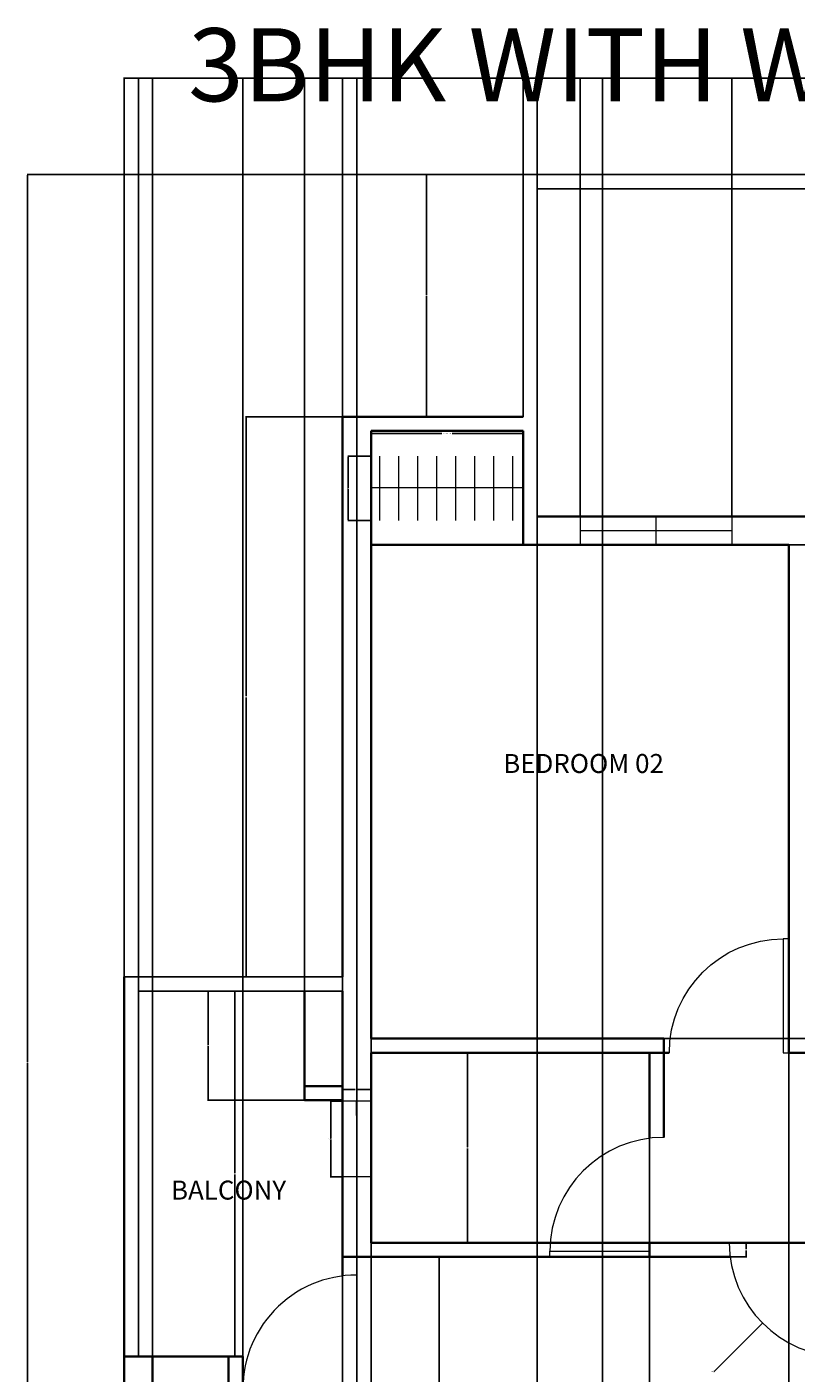
# Model space of a CAD drawing. Units: inches. Extents: x -83 to 475, y -99 to 539.
# Tile 2 of 3: x -83 to 160, y 114 to 539. Entities that reach past the tile are written whole.
import ezdxf

# ---------------------------------------------------------------- set-up
doc = ezdxf.new("R2010")
doc.units = ezdxf.units.IN
doc.header["$LTSCALE"] = 0.5
doc.header["$MEASUREMENT"] = 0
for name, color, linetype, lineweight in [('A-ANNO-DIMS', 2, 'Continuous', 18), ('A-ANNO-TEXT', 7, 'Continuous', 25), ('A-AREA-IDEN', 7, 'Continuous', 18), ('A-DOOR', 3, 'Continuous', 18), ('A-FURN', 8, 'Continuous', 13), ('A-GLAZ', 4, 'Continuous', 18), ('A-WALL', 7, 'Continuous', 35), ('A-WALL-PRPT', 7, 'Continuous', 25)]:
    doc.layers.add(name, color=color, linetype=linetype, lineweight=lineweight)
doc.styles.get("Standard").update_dxf_attribs({"font": 'arial.ttf'})
doc.dimstyles.get("Standard").update_dxf_attribs({"dimtxt": 0.18, "dimasz": 0.18, "dimexe": 0.18, "dimexo": 0.0625, "dimgap": 0.09, "dimtad": 0, "dimtih": 1, "dimtoh": 1, "dimdec": 4, "dimzin": 0, "dimdsep": 46, "dimtxsty": 'Standard', "dimcen": 0.09, "dimadec": 0, "dimazin": 0, "dimtfac": 1, "dimtdec": 4, "dimtofl": 0, "dimtmove": 0, "dimatfit": 3, "dimfxl": 1, "dimtolj": 1, "dimtzin": 0, "dimarcsym": 0})

# ---------------------------------------------------------------- blocks, each defined once
blk = doc.blocks.new('DOOR-SWING-36')
blk.add_lwpolyline([(1.78, 0), (0, 0), (0, 36.03), (1.78, 36.03)], close=True)
blk.add_arc((1.78, 0), 36, 0, 90)
blk = doc.blocks.new('WIN-48-TWO-LIGHT')
for p, q in [((0, 9), (0, 0)), ((24, 9), (24, 0)), ((48, 9), (48, 0)), ((0, 4.5), (48, 4.5))]:
    blk.add_line(p, q)
blk = doc.blocks.new('WIN-24')
for p, q in [((9, 24), (0, 24)), ((4.5, 19.41), (4.5, 24)), ((4.5, 19.41), (4.5, 0)), ((9, 0), (0, 0))]:
    blk.add_line(p, q)
blk = doc.blocks.new('WARDROBE-RAIL-48')
for p, q in [((2.64, 20.32), (2.64, 0)), ((8.64, 20.32), (8.64, 0)), ((14.64, 20.32), (14.64, 0)), ((20.64, 20.32), (20.64, 0)), ((26.64, 20.32), (26.64, 0)), ((32.64, 20.32), (32.64, 0)), ((38.64, 20.32), (38.64, 0)), ((44.64, 20.32), (44.64, 0)), ((48, 10.3), (0, 10.3))]:
    blk.add_line(p, q)
blk = doc.blocks.new('*D10')
at = {"layer": 'A-ANNO-DIMS', "color": 0, "lineweight": -2, "transparency": 16777216}
for p, q in [((16.39, 199.88), (12.67, 199.88)), ((12.85, 199.7), (12.85, 188.06)), ((12.85, 176.06), (12.85, 187.69)), ((16.39, 175.88), (12.67, 175.88))]:
    blk.add_line(p, q, dxfattribs=at)
at = {"layer": 'A-ANNO-DIMS', "color": 0, "transparency": 16777216}
for points in [[(12.82, 199.7), (12.88, 199.7), (12.85, 199.88)], [(12.82, 176.06), (12.88, 176.06), (12.85, 175.88)]]:
    blk.add_solid(points, dxfattribs=at)
at = {"layer": 'Defpoints', "color": 0, "transparency": 16777216}
for p in [(12.85, 199.88), (16.45, 199.88), (16.45, 175.88)]:
    blk.add_point(p, dxfattribs=at)
at = {"layer": 'A-ANNO-DIMS', "color": 0, "transparency": 16777216, "insert": (12.85, 187.88), "char_height": 0.18, "attachment_point": 5}
blk.add_mtext('\\A1;WINDOW 24 TYP.', dxfattribs=at)
blk = doc.blocks.new('*D11')
at = {"layer": 'A-ANNO-DIMS', "color": 0, "lineweight": -2, "transparency": 16777216}
for p, q in [((16.45, 199.94), (16.45, 203.66)), ((16.63, 203.48), (20.49, 203.48)), ((25.27, 203.48), (21.41, 203.48)), ((25.45, 199.94), (25.45, 203.66))]:
    blk.add_line(p, q, dxfattribs=at)
at = {"layer": 'A-ANNO-DIMS', "color": 0, "transparency": 16777216}
for points in [[(16.63, 203.51), (16.63, 203.45), (16.45, 203.48)], [(25.27, 203.51), (25.27, 203.45), (25.45, 203.48)]]:
    blk.add_solid(points, dxfattribs=at)
at = {"layer": 'Defpoints', "color": 0, "transparency": 16777216}
for p in [(25.45, 203.48), (16.45, 199.88), (25.45, 199.88)]:
    blk.add_point(p, dxfattribs=at)
at = {"layer": 'A-ANNO-DIMS', "color": 0, "transparency": 16777216, "insert": (20.95, 203.48), "char_height": 0.18, "attachment_point": 5}
blk.add_mtext('\\A1;9 TYP.', dxfattribs=at)
blk = doc.blocks.new('*D12')
at = {"layer": 'A-ANNO-DIMS', "color": 0, "lineweight": -2, "transparency": 16777216}
for p, q in [((25.54, 403.69), (25.54, 411.01)), ((25.72, 410.83), (47.92, 410.83)), ((73.36, 410.83), (51.16, 410.83)), ((73.54, 403.69), (73.54, 411.01))]:
    blk.add_line(p, q, dxfattribs=at)
at = {"layer": 'A-ANNO-DIMS', "color": 0, "transparency": 16777216}
for points in [[(25.72, 410.86), (25.72, 410.8), (25.54, 410.83)], [(73.36, 410.86), (73.36, 410.8), (73.54, 410.83)]]:
    blk.add_solid(points, dxfattribs=at)
at = {"layer": 'Defpoints', "color": 0, "transparency": 16777216}
for p in [(73.54, 410.83), (25.54, 403.63), (73.54, 403.63)]:
    blk.add_point(p, dxfattribs=at)
at = {"layer": 'A-ANNO-DIMS', "color": 0, "transparency": 16777216, "insert": (49.54, 410.83), "char_height": 0.18, "attachment_point": 5}
blk.add_mtext('\\A1;WARDROBE RAIL 48 TYP.', dxfattribs=at)
blk = doc.blocks.new('*D13')
at = {"layer": 'A-ANNO-DIMS', "color": 0, "lineweight": -2, "transparency": 16777216}
for p, q in [((25.48, 403.63), (18.16, 403.63)), ((18.34, 403.45), (18.34, 393.65)), ((18.34, 383.49), (18.34, 393.29)), ((25.48, 383.31), (18.16, 383.31))]:
    blk.add_line(p, q, dxfattribs=at)
at = {"layer": 'A-ANNO-DIMS', "color": 0, "transparency": 16777216}
for points in [[(18.31, 403.45), (18.37, 403.45), (18.34, 403.63)], [(18.31, 383.49), (18.37, 383.49), (18.34, 383.31)]]:
    blk.add_solid(points, dxfattribs=at)
at = {"layer": 'Defpoints', "color": 0, "transparency": 16777216}
for p in [(18.34, 403.63), (25.54, 403.63), (25.54, 383.31)]:
    blk.add_point(p, dxfattribs=at)
at = {"layer": 'A-ANNO-DIMS', "color": 0, "transparency": 16777216, "insert": (18.34, 393.47), "char_height": 0.18, "attachment_point": 5}
blk.add_mtext('\\A1;20 TYP.', dxfattribs=at)
blk = doc.blocks.new('*D15')
at = {"layer": 'A-ANNO-DIMS', "color": 0, "lineweight": -2, "transparency": 16777216}
for p, q in [((73.48, 492.61), (-83.14, 492.61)), ((-82.96, 492.43), (-82.96, 212.3)), ((-82.96, -68.21), (-82.96, 211.93)), ((214.1, -68.39), (-83.14, -68.39))]:
    blk.add_line(p, q, dxfattribs=at)
at = {"layer": 'A-ANNO-DIMS', "color": 0, "transparency": 16777216}
for points in [[(-82.99, 492.43), (-82.93, 492.43), (-82.96, 492.61)], [(-82.99, -68.21), (-82.93, -68.21), (-82.96, -68.39)]]:
    blk.add_solid(points, dxfattribs=at)
at = {"layer": 'Defpoints', "color": 0, "transparency": 16777216}
for p in [(-82.96, 492.61), (73.54, 492.61), (214.16, -68.39)]:
    blk.add_point(p, dxfattribs=at)
at = {"layer": 'A-ANNO-DIMS', "color": 0, "transparency": 16777216, "insert": (-82.96, 212.11), "char_height": 0.18, "attachment_point": 5}
blk.add_mtext('\\A1;561', dxfattribs=at)
blk = doc.blocks.new('*D16')
at = {"layer": 'A-ANNO-DIMS', "color": 0, "lineweight": -2, "transparency": 16777216}
for p, q in [((78.04, 488.05), (78.04, -99.07)), ((294.04, 488.05), (294.04, -99.07)), ((78.22, -98.89), (185.75, -98.89)), ((293.86, -98.89), (186.33, -98.89))]:
    blk.add_line(p, q, dxfattribs=at)
at = {"layer": 'A-ANNO-DIMS', "color": 0, "transparency": 16777216}
for points in [[(78.22, -98.86), (78.22, -98.92), (78.04, -98.89)], [(293.86, -98.86), (293.86, -98.92), (294.04, -98.89)]]:
    blk.add_solid(points, dxfattribs=at)
at = {"layer": 'Defpoints', "color": 0, "transparency": 16777216}
for p in [(78.04, 488.11), (294.04, 488.11), (294.04, -98.89)]:
    blk.add_point(p, dxfattribs=at)
at = {"layer": 'A-ANNO-DIMS', "color": 0, "transparency": 16777216, "insert": (186.04, -98.89), "char_height": 0.18, "attachment_point": 5}
blk.add_mtext('\\A1;216', dxfattribs=at)
blk = doc.blocks.new('*D18')
at = {"layer": 'A-ANNO-DIMS', "color": 0, "lineweight": -2, "transparency": 16777216}
for p, q in [((73.48, 492.61), (42.86, 492.61)), ((43.04, 492.43), (43.04, 454.55)), ((43.04, 416.29), (43.04, 454.18)), ((73.48, 416.11), (42.86, 416.11))]:
    blk.add_line(p, q, dxfattribs=at)
at = {"layer": 'A-ANNO-DIMS', "color": 0, "transparency": 16777216}
for points in [[(43.01, 492.43), (43.07, 492.43), (43.04, 492.61)], [(43.01, 416.29), (43.07, 416.29), (43.04, 416.11)]]:
    blk.add_solid(points, dxfattribs=at)
at = {"layer": 'Defpoints', "color": 0, "transparency": 16777216}
for p in [(43.04, 492.61), (73.54, 492.61), (73.54, 416.11)]:
    blk.add_point(p, dxfattribs=at)
at = {"layer": 'A-ANNO-DIMS', "color": 0, "transparency": 16777216, "insert": (43.04, 454.36), "char_height": 0.18, "attachment_point": 5}
blk.add_mtext('\\A1;76.5', dxfattribs=at)
blk = doc.blocks.new('*D19')
at = {"layer": 'A-ANNO-DIMS', "color": 0, "lineweight": -2, "transparency": 16777216}
for p, q in [((25.54, 375.55), (25.54, -99.07)), ((157.54, 375.55), (157.54, -99.07)), ((25.72, -98.89), (91.26, -98.89)), ((157.36, -98.89), (91.82, -98.89))]:
    blk.add_line(p, q, dxfattribs=at)
at = {"layer": 'A-ANNO-DIMS', "color": 0, "transparency": 16777216}
for points in [[(25.72, -98.86), (25.72, -98.92), (25.54, -98.89)], [(157.36, -98.86), (157.36, -98.92), (157.54, -98.89)]]:
    blk.add_solid(points, dxfattribs=at)
at = {"layer": 'Defpoints', "color": 0, "transparency": 16777216}
for p in [(25.54, 375.61), (157.54, 375.61), (157.54, -98.89)]:
    blk.add_point(p, dxfattribs=at)
at = {"layer": 'A-ANNO-DIMS', "color": 0, "transparency": 16777216, "insert": (91.54, -98.89), "char_height": 0.18, "attachment_point": 5}
blk.add_mtext('\\A1;132', dxfattribs=at)
blk = doc.blocks.new('*D21')
at = {"layer": 'A-ANNO-DIMS', "color": 0, "lineweight": -2, "transparency": 16777216}
for p, q in [((25.6, 375.61), (474.72, 375.61)), ((474.54, 375.43), (474.54, 297.8)), ((474.54, 219.79), (474.54, 297.43)), ((25.6, 219.61), (474.72, 219.61))]:
    blk.add_line(p, q, dxfattribs=at)
at = {"layer": 'A-ANNO-DIMS', "color": 0, "transparency": 16777216}
for points in [[(474.51, 375.43), (474.57, 375.43), (474.54, 375.61)], [(474.51, 219.79), (474.57, 219.79), (474.54, 219.61)]]:
    blk.add_solid(points, dxfattribs=at)
at = {"layer": 'Defpoints', "color": 0, "transparency": 16777216}
for p in [(25.54, 375.61), (474.54, 375.61), (25.54, 219.61)]:
    blk.add_point(p, dxfattribs=at)
at = {"layer": 'A-ANNO-DIMS', "color": 0, "transparency": 16777216, "insert": (474.54, 297.61), "char_height": 0.18, "attachment_point": 5}
blk.add_mtext('\\A1;156', dxfattribs=at)
blk = doc.blocks.new('*D29')
at = {"layer": 'A-ANNO-DIMS', "color": 0, "lineweight": -2, "transparency": 16777216}
for p, q in [((-52.46, 239.18), (-52.46, 523.29)), ((16.54, 239.18), (16.54, 523.29)), ((-52.28, 523.11), (-18.18, 523.11)), ((16.36, 523.11), (-17.74, 523.11))]:
    blk.add_line(p, q, dxfattribs=at)
at = {"layer": 'A-ANNO-DIMS', "color": 0, "transparency": 16777216}
for points in [[(-52.28, 523.14), (-52.28, 523.08), (-52.46, 523.11)], [(16.36, 523.14), (16.36, 523.08), (16.54, 523.11)]]:
    blk.add_solid(points, dxfattribs=at)
at = {"layer": 'Defpoints', "color": 0, "transparency": 16777216}
for p in [(16.54, 523.11), (-52.46, 239.11), (16.54, 239.11)]:
    blk.add_point(p, dxfattribs=at)
at = {"layer": 'A-ANNO-DIMS', "color": 0, "transparency": 16777216, "insert": (-17.96, 523.11), "char_height": 0.18, "attachment_point": 5}
blk.add_mtext('\\A1;69', dxfattribs=at)
blk = doc.blocks.new('*D30')
at = {"layer": 'A-ANNO-DIMS', "color": 0, "lineweight": -2, "transparency": 16777216}
for p, q in [((16.48, 416.11), (-14.14, 416.11)), ((-13.96, 415.93), (-13.96, 327.79)), ((-13.96, 239.29), (-13.96, 327.43)), ((16.48, 239.11), (-14.14, 239.11))]:
    blk.add_line(p, q, dxfattribs=at)
at = {"layer": 'A-ANNO-DIMS', "color": 0, "transparency": 16777216}
for points in [[(-13.99, 415.93), (-13.93, 415.93), (-13.96, 416.11)], [(-13.99, 239.29), (-13.93, 239.29), (-13.96, 239.11)]]:
    blk.add_solid(points, dxfattribs=at)
at = {"layer": 'Defpoints', "color": 0, "transparency": 16777216}
for p in [(-13.96, 416.11), (16.54, 416.11), (16.54, 239.11)]:
    blk.add_point(p, dxfattribs=at)
at = {"layer": 'A-ANNO-DIMS', "color": 0, "transparency": 16777216, "insert": (-13.96, 327.61), "char_height": 0.18, "attachment_point": 5}
blk.add_mtext('\\A1;177', dxfattribs=at)
blk = doc.blocks.new('*D31')
at = {"layer": 'A-ANNO-DIMS', "color": 0, "lineweight": -2, "transparency": 16777216}
for p, q in [((-47.9, 234.61), (-17.28, 234.61)), ((-17.46, 234.43), (-17.46, 177.05)), ((-17.46, 119.29), (-17.46, 176.68)), ((-47.9, 119.11), (-17.28, 119.11))]:
    blk.add_line(p, q, dxfattribs=at)
at = {"layer": 'A-ANNO-DIMS', "color": 0, "transparency": 16777216}
for points in [[(-17.49, 234.43), (-17.43, 234.43), (-17.46, 234.61)], [(-17.49, 119.29), (-17.43, 119.29), (-17.46, 119.11)]]:
    blk.add_solid(points, dxfattribs=at)
at = {"layer": 'Defpoints', "color": 0, "transparency": 16777216}
for p in [(-47.96, 234.61), (-47.96, 119.11), (-17.46, 119.11)]:
    blk.add_point(p, dxfattribs=at)
at = {"layer": 'A-ANNO-DIMS', "color": 0, "transparency": 16777216, "insert": (-17.46, 176.86), "char_height": 0.18, "attachment_point": 5}
blk.add_mtext('\\A1;115.5', dxfattribs=at)
blk = doc.blocks.new('*D32')
at = {"layer": 'A-ANNO-DIMS', "color": 0, "lineweight": -2, "transparency": 16777216}
for p, q in [((25.6, 215.11), (56.22, 215.11)), ((56.04, 214.93), (56.04, 185.3)), ((56.04, 155.29), (56.04, 184.93)), ((25.6, 155.11), (56.22, 155.11))]:
    blk.add_line(p, q, dxfattribs=at)
at = {"layer": 'A-ANNO-DIMS', "color": 0, "transparency": 16777216}
for points in [[(56.01, 214.93), (56.07, 214.93), (56.04, 215.11)], [(56.01, 155.29), (56.07, 155.29), (56.04, 155.11)]]:
    blk.add_solid(points, dxfattribs=at)
at = {"layer": 'Defpoints', "color": 0, "transparency": 16777216}
for p in [(25.54, 215.11), (25.54, 155.11), (56.04, 155.11)]:
    blk.add_point(p, dxfattribs=at)
at = {"layer": 'A-ANNO-DIMS', "color": 0, "transparency": 16777216, "insert": (56.04, 185.11), "char_height": 0.18, "attachment_point": 5}
blk.add_mtext('\\A1;60', dxfattribs=at)
blk = doc.blocks.new('*D33')
at = {"layer": 'A-ANNO-DIMS', "color": 0, "lineweight": -2, "transparency": 16777216}
for p, q in [((25.54, 215.05), (25.54, -99.07)), ((113.54, 215.05), (113.54, -99.07)), ((25.72, -98.89), (69.32, -98.89)), ((113.36, -98.89), (69.76, -98.89))]:
    blk.add_line(p, q, dxfattribs=at)
at = {"layer": 'A-ANNO-DIMS', "color": 0, "transparency": 16777216}
for points in [[(25.72, -98.86), (25.72, -98.92), (25.54, -98.89)], [(113.36, -98.86), (113.36, -98.92), (113.54, -98.89)]]:
    blk.add_solid(points, dxfattribs=at)
at = {"layer": 'Defpoints', "color": 0, "transparency": 16777216}
for p in [(25.54, 215.11), (113.54, 215.11), (113.54, -98.89)]:
    blk.add_point(p, dxfattribs=at)
at = {"layer": 'A-ANNO-DIMS', "color": 0, "transparency": 16777216, "insert": (69.54, -98.89), "char_height": 0.18, "attachment_point": 5}
blk.add_mtext('\\A1;88', dxfattribs=at)
blk = doc.blocks.new('*D34')
at = {"layer": 'A-ANNO-DIMS', "color": 0, "lineweight": -2, "transparency": 16777216}
for p, q in [((113.6, 155.11), (144.22, 155.11)), ((144.04, 154.93), (144.04, 153.05)), ((113.6, 150.61), (144.22, 150.61)), ((144.04, 150.79), (144.04, 152.68))]:
    blk.add_line(p, q, dxfattribs=at)
at = {"layer": 'A-ANNO-DIMS', "color": 0, "transparency": 16777216}
for points in [[(144.01, 154.93), (144.07, 154.93), (144.04, 155.11)], [(144.01, 150.79), (144.07, 150.79), (144.04, 150.61)]]:
    blk.add_solid(points, dxfattribs=at)
at = {"layer": 'Defpoints', "color": 0, "transparency": 16777216}
for p in [(113.54, 155.11), (113.54, 150.61), (144.04, 150.61)]:
    blk.add_point(p, dxfattribs=at)
at = {"layer": 'A-ANNO-DIMS', "color": 0, "transparency": 16777216, "insert": (144.04, 152.86), "char_height": 0.18, "attachment_point": 5}
blk.add_mtext('\\A1;4.5', dxfattribs=at)
blk = doc.blocks.new('*D35')
at = {"layer": 'A-ANNO-DIMS', "color": 0, "lineweight": -2, "transparency": 16777216}
for p, q in [((21.04, 18.68), (21.04, 523.29)), ((214.16, 18.68), (214.16, 523.29)), ((21.22, 523.11), (117.15, 523.11)), ((213.98, 523.11), (118.05, 523.11))]:
    blk.add_line(p, q, dxfattribs=at)
at = {"layer": 'A-ANNO-DIMS', "color": 0, "transparency": 16777216}
for points in [[(21.22, 523.14), (21.22, 523.08), (21.04, 523.11)], [(213.98, 523.14), (213.98, 523.08), (214.16, 523.11)]]:
    blk.add_solid(points, dxfattribs=at)
at = {"layer": 'Defpoints', "color": 0, "transparency": 16777216}
for p in [(214.16, 523.11), (21.04, 18.61), (214.16, 18.61)]:
    blk.add_point(p, dxfattribs=at)
at = {"layer": 'A-ANNO-DIMS', "color": 0, "transparency": 16777216, "insert": (117.6, 523.11), "char_height": 0.18, "attachment_point": 5}
blk.add_mtext('\\A1;193.12', dxfattribs=at)
blk = doc.blocks.new('*D36')
at = {"layer": 'A-ANNO-DIMS', "color": 0, "lineweight": -2, "transparency": 16777216}
for p, q in [((16.6, 150.61), (47.22, 150.61)), ((47.04, 150.43), (47.04, 84.8)), ((47.04, 18.79), (47.04, 84.43)), ((16.6, 18.61), (47.22, 18.61))]:
    blk.add_line(p, q, dxfattribs=at)
at = {"layer": 'A-ANNO-DIMS', "color": 0, "transparency": 16777216}
for points in [[(47.01, 150.43), (47.07, 150.43), (47.04, 150.61)], [(47.01, 18.79), (47.07, 18.79), (47.04, 18.61)]]:
    blk.add_solid(points, dxfattribs=at)
at = {"layer": 'Defpoints', "color": 0, "transparency": 16777216}
for p in [(16.54, 150.61), (16.54, 18.61), (47.04, 18.61)]:
    blk.add_point(p, dxfattribs=at)
at = {"layer": 'A-ANNO-DIMS', "color": 0, "transparency": 16777216, "insert": (47.04, 84.61), "char_height": 0.18, "attachment_point": 5}
blk.add_mtext('\\A1;132', dxfattribs=at)
blk = doc.blocks.new('*D37')
at = {"layer": 'A-ANNO-DIMS', "color": 0, "lineweight": -2, "transparency": 16777216}
for p, q in [((-43.46, 18.68), (-43.46, 523.29)), ((16.54, 18.68), (16.54, 523.29)), ((-43.28, 523.11), (-13.68, 523.11)), ((16.36, 523.11), (-13.24, 523.11))]:
    blk.add_line(p, q, dxfattribs=at)
at = {"layer": 'A-ANNO-DIMS', "color": 0, "transparency": 16777216}
for points in [[(-43.28, 523.14), (-43.28, 523.08), (-43.46, 523.11)], [(16.36, 523.14), (16.36, 523.08), (16.54, 523.11)]]:
    blk.add_solid(points, dxfattribs=at)
at = {"layer": 'Defpoints', "color": 0, "transparency": 16777216}
for p in [(16.54, 523.11), (-43.46, 18.61), (16.54, 18.61)]:
    blk.add_point(p, dxfattribs=at)
at = {"layer": 'A-ANNO-DIMS', "color": 0, "transparency": 16777216, "insert": (-13.46, 523.11), "char_height": 0.18, "attachment_point": 5}
blk.add_mtext('\\A1;60', dxfattribs=at)
blk = doc.blocks.new('*D47')
at = {"layer": 'A-ANNO-DIMS', "color": 0, "lineweight": -2, "transparency": 16777216}
for p, q in [((98.66, -45.82), (98.66, 523.29)), ((191.66, -45.82), (191.66, 523.29)), ((98.84, 523.11), (144.94, 523.11)), ((191.48, 523.11), (145.38, 523.11))]:
    blk.add_line(p, q, dxfattribs=at)
at = {"layer": 'A-ANNO-DIMS', "color": 0, "transparency": 16777216}
for points in [[(98.84, 523.14), (98.84, 523.08), (98.66, 523.11)], [(191.48, 523.14), (191.48, 523.08), (191.66, 523.11)]]:
    blk.add_solid(points, dxfattribs=at)
at = {"layer": 'Defpoints', "color": 0, "transparency": 16777216}
for p in [(191.66, 523.11), (98.66, -45.89), (191.66, -45.89)]:
    blk.add_point(p, dxfattribs=at)
at = {"layer": 'A-ANNO-DIMS', "color": 0, "transparency": 16777216, "insert": (145.16, 523.11), "char_height": 0.18, "attachment_point": 5}
blk.add_mtext('\\A1;93', dxfattribs=at)
blk = doc.blocks.new('*D51')
at = {"layer": 'A-ANNO-DIMS', "color": 0, "lineweight": -2, "transparency": 16777216}
for p, q in [((16.54, 416.18), (16.54, 523.29)), ((73.54, 416.18), (73.54, 523.29)), ((16.72, 523.11), (44.82, 523.11)), ((73.36, 523.11), (45.26, 523.11))]:
    blk.add_line(p, q, dxfattribs=at)
at = {"layer": 'A-ANNO-DIMS', "color": 0, "transparency": 16777216}
for points in [[(16.72, 523.14), (16.72, 523.08), (16.54, 523.11)], [(73.36, 523.14), (73.36, 523.08), (73.54, 523.11)]]:
    blk.add_solid(points, dxfattribs=at)
at = {"layer": 'Defpoints', "color": 0, "transparency": 16777216}
for p in [(73.54, 523.11), (16.54, 416.11), (73.54, 416.11)]:
    blk.add_point(p, dxfattribs=at)
at = {"layer": 'A-ANNO-DIMS', "color": 0, "transparency": 16777216, "insert": (45.04, 523.11), "char_height": 0.18, "attachment_point": 5}
blk.add_mtext('\\A1;57', dxfattribs=at)
blk = doc.blocks.new('*D52')
at = {"layer": 'A-ANNO-DIMS', "color": 0, "lineweight": -2, "transparency": 16777216}
for p, q in [((78.04, 384.68), (78.04, 523.29)), ((91.54, 384.68), (91.54, 523.29)), ((78.22, 523.11), (84.47, 523.11)), ((91.36, 523.11), (85.11, 523.11))]:
    blk.add_line(p, q, dxfattribs=at)
at = {"layer": 'A-ANNO-DIMS', "color": 0, "transparency": 16777216}
for points in [[(78.22, 523.14), (78.22, 523.08), (78.04, 523.11)], [(91.36, 523.14), (91.36, 523.08), (91.54, 523.11)]]:
    blk.add_solid(points, dxfattribs=at)
at = {"layer": 'Defpoints', "color": 0, "transparency": 16777216}
for p in [(91.54, 523.11), (78.04, 384.61), (91.54, 384.61)]:
    blk.add_point(p, dxfattribs=at)
at = {"layer": 'A-ANNO-DIMS', "color": 0, "transparency": 16777216, "insert": (84.79, 523.11), "char_height": 0.18, "attachment_point": 5}
blk.add_mtext('\\A1;13.5', dxfattribs=at)
blk = doc.blocks.new('*D53')
at = {"layer": 'A-ANNO-DIMS', "color": 0, "lineweight": -2, "transparency": 16777216}
for p, q in [((139.54, 384.68), (139.54, 523.29)), ((195.82, 384.62), (195.82, 523.29)), ((139.72, 523.11), (167.29, 523.11)), ((195.64, 523.11), (168.08, 523.11))]:
    blk.add_line(p, q, dxfattribs=at)
at = {"layer": 'A-ANNO-DIMS', "color": 0, "transparency": 16777216}
for points in [[(139.72, 523.14), (139.72, 523.08), (139.54, 523.11)], [(195.64, 523.14), (195.64, 523.08), (195.82, 523.11)]]:
    blk.add_solid(points, dxfattribs=at)
at = {"layer": 'Defpoints', "color": 0, "transparency": 16777216}
for p in [(195.82, 523.11), (139.54, 384.61), (195.82, 384.56)]:
    blk.add_point(p, dxfattribs=at)
at = {"layer": 'A-ANNO-DIMS', "color": 0, "transparency": 16777216, "insert": (167.68, 523.11), "char_height": 0.18, "attachment_point": 5}
blk.add_mtext('\\A1;56.28', dxfattribs=at)
blk = doc.blocks.new('*D55')
at = {"layer": 'A-ANNO-DIMS', "color": 0, "lineweight": -2, "transparency": 16777216}
for p, q in [((4.48, 234.61), (-26.14, 234.61)), ((-25.96, 234.43), (-25.96, 217.55)), ((-25.96, 200.29), (-25.96, 217.18)), ((4.48, 200.11), (-26.14, 200.11))]:
    blk.add_line(p, q, dxfattribs=at)
at = {"layer": 'A-ANNO-DIMS', "color": 0, "transparency": 16777216}
for points in [[(-25.99, 234.43), (-25.93, 234.43), (-25.96, 234.61)], [(-25.99, 200.29), (-25.93, 200.29), (-25.96, 200.11)]]:
    blk.add_solid(points, dxfattribs=at)
at = {"layer": 'Defpoints', "color": 0, "transparency": 16777216}
for p in [(-25.96, 234.61), (4.54, 234.61), (4.54, 200.11)]:
    blk.add_point(p, dxfattribs=at)
at = {"layer": 'A-ANNO-DIMS', "color": 0, "transparency": 16777216, "insert": (-25.96, 217.36), "char_height": 0.18, "attachment_point": 5}
blk.add_mtext('\\A1;34.5', dxfattribs=at)
blk = doc.blocks.new('*D56')
at = {"layer": 'A-ANNO-DIMS', "color": 0, "lineweight": -2, "transparency": 16777216}
for p, q in [((4.54, 200.18), (4.54, 523.29)), ((16.54, 200.18), (16.54, 523.29)), ((4.72, 523.11), (10.33, 523.11)), ((16.36, 523.11), (10.75, 523.11))]:
    blk.add_line(p, q, dxfattribs=at)
at = {"layer": 'A-ANNO-DIMS', "color": 0, "transparency": 16777216}
for points in [[(4.72, 523.14), (4.72, 523.08), (4.54, 523.11)], [(16.36, 523.14), (16.36, 523.08), (16.54, 523.11)]]:
    blk.add_solid(points, dxfattribs=at)
at = {"layer": 'Defpoints', "color": 0, "transparency": 16777216}
for p in [(16.54, 523.11), (4.54, 200.11), (16.54, 200.11)]:
    blk.add_point(p, dxfattribs=at)
at = {"layer": 'A-ANNO-DIMS', "color": 0, "transparency": 16777216, "insert": (10.54, 523.11), "char_height": 0.18, "attachment_point": 5}
blk.add_mtext('\\A1;12', dxfattribs=at)
blk = doc.blocks.new('*D57')
at = {"layer": 'A-ANNO-DIMS', "color": 0, "lineweight": -2, "transparency": 16777216}
for p, q in [((-47.96, 119.18), (-47.96, 523.29)), ((-14.96, 119.18), (-14.96, 523.29)), ((-47.78, 523.11), (-31.68, 523.11)), ((-15.14, 523.11), (-31.24, 523.11))]:
    blk.add_line(p, q, dxfattribs=at)
at = {"layer": 'A-ANNO-DIMS', "color": 0, "transparency": 16777216}
for points in [[(-47.78, 523.14), (-47.78, 523.08), (-47.96, 523.11)], [(-15.14, 523.14), (-15.14, 523.08), (-14.96, 523.11)]]:
    blk.add_solid(points, dxfattribs=at)
at = {"layer": 'Defpoints', "color": 0, "transparency": 16777216}
for p in [(-14.96, 523.11), (-47.96, 119.11), (-14.96, 119.11)]:
    blk.add_point(p, dxfattribs=at)
at = {"layer": 'A-ANNO-DIMS', "color": 0, "transparency": 16777216, "insert": (-31.46, 523.11), "char_height": 0.18, "attachment_point": 5}
blk.add_mtext('\\A1;33', dxfattribs=at)
blk = doc.blocks.new('*D62')
at = {"layer": 'A-ANNO-DIMS', "color": 0, "lineweight": -2, "transparency": 16777216}
for p, q in [((174.61, 155.11), (174.79, 155.11)), ((174.7, 155.02), (174.7, 155.2)), ((133.97, 114.38), (149.11, 129.53)), ((133.79, 114.38), (133.97, 114.38))]:
    blk.add_line(p, q, dxfattribs=at)
at = {"layer": 'A-ANNO-DIMS', "color": 0, "transparency": 16777216}
blk.add_solid([(149.09, 129.55), (149.13, 129.51), (149.24, 129.66)], dxfattribs=at)
at = {"layer": 'Defpoints', "color": 0, "transparency": 16777216}
for p in [(174.7, 155.11), (149.24, 129.66)]:
    blk.add_point(p, dxfattribs=at)
at = {"layer": 'A-ANNO-DIMS', "color": 0, "transparency": 16777216, "insert": (133.29, 114.38), "char_height": 0.18, "attachment_point": 5}
blk.add_mtext('\\A1;6X R36', dxfattribs=at)

msp = doc.modelspace()

# ---------------------------------------------------------------- linework, layer by layer
at = {"layer": 'A-DOOR'}
msp.add_lwpolyline([(118.04, 150.614), (118.04, 150.614), (82.012, 150.614), (82.012, 152.398), (113.54, 152.398)], dxfattribs=at)
for centre, start, end in [((118.04, 152.398), 90, 180), ((174.697, 155.114), 180, 270), ((21.04, 108.898), 90, 182.84057)]:
    msp.add_arc(centre, 36, start, end, dxfattribs=at)
at = {"layer": 'A-WALL'}
for p, q in [((16.54, 416.114), (73.54, 416.114)), ((16.54, 239.114), (16.54, 416.114)), ((16.54, 239.114), (16.54, 416.114)), ((25.54, 411.614), (73.54, 411.614)), ((25.54, 219.614), (25.54, 411.614)), ((73.54, 375.614), (73.54, 411.614)), ((78.04, 384.614), (294.04, 384.614)), ((25.54, 375.614), (157.54, 375.614)), ((157.54, 215.114), (157.54, 375.614)), ((-52.46, 9.614), (-52.46, 239.114)), ((4.54, 200.114), (4.54, 234.614)), ((16.54, 144.616), (16.54, 234.614)), ((16.54, 144.616), (16.54, 234.614)), ((25.54, 219.614), (118.04, 219.614)), ((118.04, 188.398), (118.04, 219.614)), ((25.54, 155.114), (25.54, 215.114)), ((25.54, 215.114), (119.756, 215.114)), ((113.54, 188.116), (113.54, 215.114)), ((157.54, 215.114), (163.824, 215.114)), ((16.54, 204.614), (4.54, 204.614)), ((16.54, 200.114), (4.54, 200.114)), ((25.54, 155.114), (113.54, 155.114)), ((113.54, 150.614), (113.54, 155.114)), ((113.54, 155.114), (180.981, 155.114)), ((16.54, 150.614), (138.979, 150.614)), ((-14.96, 119.114), (-52.46, 119.114)), ((-43.46, 107.114), (-43.46, 119.114)), ((-19.46, 107.114), (-19.46, 119.114)), ((-14.96, 107.114), (-14.96, 119.114))]:
    msp.add_line(p, q, dxfattribs=at)
at = {"layer": 'A-WALL-PRPT'}
for p, q in [((73.54, 492.614), (298.54, 492.614)), ((73.54, 416.114), (73.54, 492.614)), ((78.04, 384.614), (78.04, 488.114)), ((78.04, 488.114), (294.04, 488.114)), ((16.54, 239.114), (-52.46, 239.114)), ((16.54, 234.614), (-47.96, 234.614)), ((-47.96, 119.114), (-47.96, 234.614))]:
    msp.add_line(p, q, dxfattribs=at)

# ---------------------------------------------------------------- block references
at = {"layer": 'A-DOOR', "extrusion": (0, 0, -1), "zscale": -1}
msp.add_blockref('DOOR-SWING-36', (-157.54, 215.114), dxfattribs=at)
at = {"layer": 'A-FURN'}
msp.add_blockref('WARDROBE-RAIL-48', (25.54, 383.31), dxfattribs=at)
at = {"layer": 'A-GLAZ'}
for name, p in [('WIN-48-TWO-LIGHT', (91.54, 375.614)), ('WIN-24', (16.451, 175.877))]:
    msp.add_blockref(name, p, dxfattribs=at)

# ---------------------------------------------------------------- texts
at = {"layer": 'A-ANNO-TEXT', "insert": (-32.222, 538.87), "char_height": 23.10502, "attachment_point": 1}
msp.add_mtext_dynamic_manual_height_columns('3BHK WITH WIDE BALCONY', width=1678.41017, gutter_width=115.525, heights=[0], dxfattribs=at)
at = {"layer": 'A-AREA-IDEN'}
for s, p in [(' BEDROOM 02', (65.457, 303.532)), ('BALCONY', (-37.647, 168.731))]:
    msp.add_text(s, height=6, dxfattribs=at).set_placement(p)

# ---------------------------------------------------------------- dimensions: what is measured, and where the dimension line sits
at = {"layer": 'A-ANNO-DIMS'}
for base, p1, p2, override, picture, middle in [((16.54, 523.114), (-52.46, 239.114), (16.54, 239.114), {"dimdec": 0, "dimlfac": 1, "dimrnd": 0, "dimzin": 0, "dimdsep": 46, "dimlunit": 2}, '*D29', (-17.96, 523.114)), ((-14.96, 523.114), (-47.96, 119.114), (-14.96, 119.114), {"dimdec": 0, "dimlfac": 1, "dimrnd": 0, "dimzin": 0, "dimdsep": 46, "dimlunit": 2}, '*D57', (-31.46, 523.114)), ((16.54, 523.114), (-43.46, 18.614), (16.54, 18.614), {"dimdec": 0, "dimlfac": 1, "dimrnd": 0, "dimzin": 0, "dimdsep": 46, "dimlunit": 2}, '*D37', (-13.46, 523.114)), ((16.54, 523.114), (4.54, 200.114), (16.54, 200.114), {"dimdec": 0, "dimlfac": 1, "dimrnd": 0, "dimzin": 0, "dimdsep": 46, "dimlunit": 2}, '*D56', (10.54, 523.114)), ((73.54, 523.114), (16.54, 416.114), (73.54, 416.114), {"dimdec": 0, "dimlfac": 1, "dimrnd": 0, "dimzin": 0, "dimdsep": 46, "dimlunit": 2}, '*D51', (45.04, 523.114)), ((214.161, 523.114), (21.04, 18.614), (214.161, 18.614), {"dimdec": 2, "dimlfac": 1, "dimrnd": 0, "dimzin": 0, "dimdsep": 46, "dimlunit": 2}, '*D35', (117.601, 523.114)), ((91.54, 523.114), (78.04, 384.614), (91.54, 384.614), {"dimdec": 1, "dimlfac": 1, "dimrnd": 0, "dimzin": 0, "dimdsep": 46, "dimlunit": 2}, '*D52', (84.79, 523.114)), ((191.661, 523.114), (98.661, -45.886), (191.661, -45.886), {"dimdec": 0, "dimlfac": 1, "dimrnd": 0, "dimzin": 0, "dimdsep": 46, "dimlunit": 2}, '*D47', (145.161, 523.114)), ((195.824, 523.114), (139.54, 384.614), (195.824, 384.561), {"dimdec": 2, "dimlfac": 1, "dimrnd": 0, "dimzin": 0, "dimdsep": 46, "dimlunit": 2}, '*D53', (167.682, 523.114)), ((294.04, -98.886), (78.04, 488.114), (294.04, 488.114), {"dimdec": 0, "dimlfac": 1, "dimrnd": 0, "dimzin": 0, "dimdsep": 46, "dimlunit": 2}, '*D16', (186.04, -98.886)), ((157.54, -98.886), (25.54, 375.614), (157.54, 375.614), {"dimdec": 0, "dimlfac": 1, "dimrnd": 0, "dimzin": 0, "dimdsep": 46, "dimlunit": 2}, '*D19', (91.54, -98.886)), ((113.54, -98.886), (25.54, 215.114), (113.54, 215.114), {"dimdec": 0, "dimlfac": 1, "dimrnd": 0, "dimzin": 0, "dimdsep": 46, "dimlunit": 2}, '*D33', (69.54, -98.886))]:
    dim = msp.add_linear_dim(base=base, p1=p1, p2=p2, dimstyle='Standard', override=override, dxfattribs=at)
    dim.commit()
    dim.dimension.update_dxf_attribs({"geometry": picture, "text_midpoint": middle})
for base, p1, p2, angle, override, picture, middle in [((-82.96, 492.614), (214.161, -68.386), (73.54, 492.614), 90, {"dimdec": 0, "dimlfac": 1, "dimrnd": 0, "dimzin": 0, "dimdsep": 46, "dimlunit": 2}, '*D15', (-82.96, 212.114)), ((43.04, 492.614), (73.54, 416.114), (73.54, 492.614), 90, {"dimdec": 1, "dimlfac": 1, "dimrnd": 0, "dimzin": 0, "dimdsep": 46, "dimlunit": 2}, '*D18', (43.04, 454.364)), ((-13.96, 416.114), (16.54, 239.114), (16.54, 416.114), 90, {"dimdec": 0, "dimlfac": 1, "dimrnd": 0, "dimzin": 0, "dimdsep": 46, "dimlunit": 2}, '*D30', (-13.96, 327.614)), ((474.54, 375.614), (25.54, 219.614), (25.54, 375.614), 90, {"dimdec": 0, "dimlfac": 1, "dimrnd": 0, "dimzin": 0, "dimdsep": 46, "dimlunit": 2}, '*D21', (474.54, 297.614)), ((-17.46, 119.114), (-47.96, 234.614), (-47.96, 119.114), 270, {"dimdec": 1, "dimlfac": 1, "dimrnd": 0, "dimzin": 0, "dimdsep": 46, "dimlunit": 2}, '*D31', (-17.46, 176.864)), ((-25.96, 234.614), (4.54, 200.114), (4.54, 234.614), 90, {"dimdec": 1, "dimlfac": 1, "dimrnd": 0, "dimzin": 0, "dimdsep": 46, "dimlunit": 2}, '*D55', (-25.96, 217.364)), ((56.04, 155.114), (25.54, 215.114), (25.54, 155.114), 270, {"dimdec": 0, "dimlfac": 1, "dimrnd": 0, "dimzin": 0, "dimdsep": 46, "dimlunit": 2}, '*D32', (56.04, 185.114)), ((144.04, 150.614), (113.54, 155.114), (113.54, 150.614), 270, {"dimdec": 1, "dimlfac": 1, "dimrnd": 0, "dimzin": 0, "dimdsep": 46, "dimlunit": 2}, '*D34', (144.04, 152.864)), ((47.04, 18.614), (16.54, 150.614), (16.54, 18.614), 270, {"dimdec": 0, "dimlfac": 1, "dimrnd": 0, "dimzin": 0, "dimdsep": 46, "dimlunit": 2}, '*D36', (47.04, 84.614))]:
    dim = msp.add_linear_dim(base=base, p1=p1, p2=p2, angle=angle, dimstyle='Standard', override=override, dxfattribs=at)
    dim.commit()
    dim.dimension.update_dxf_attribs({"geometry": picture, "text_midpoint": middle})
for base, p1, p2, text, picture, middle in [((73.54, 410.832), (25.54, 403.632), (73.54, 403.632), 'WARDROBE RAIL <> TYP.', '*D12', (49.54, 410.832)), ((25.451, 203.477), (16.451, 199.877), (25.451, 199.877), '<> TYP.', '*D11', (20.951, 203.477))]:
    dim = msp.add_linear_dim(base=base, p1=p1, p2=p2, text=text, dimstyle='Standard', override={"dimdec": 0, "dimlfac": 1, "dimrnd": 0, "dimzin": 0, "dimdsep": 46, "dimlunit": 2}, dxfattribs=at)
    dim.commit()
    dim.dimension.update_dxf_attribs({"geometry": picture, "text_midpoint": middle})
for base, p1, p2, text, picture, middle in [((18.34, 403.632), (25.54, 383.31), (25.54, 403.632), '<> TYP.', '*D13', (18.34, 393.471)), ((12.851, 199.877), (16.451, 175.877), (16.451, 199.877), 'WINDOW <> TYP.', '*D10', (12.851, 187.877))]:
    dim = msp.add_linear_dim(base=base, p1=p1, p2=p2, angle=90, text=text, dimstyle='Standard', override={"dimdec": 0, "dimlfac": 1, "dimrnd": 0, "dimzin": 0, "dimdsep": 46, "dimlunit": 2}, dxfattribs=at)
    dim.commit()
    dim.dimension.update_dxf_attribs({"geometry": picture, "text_midpoint": middle})
dim = msp.add_radius_dim(center=(174.697, 155.114), mpoint=(149.241, 129.658), text='6X <>', dimstyle='Standard', override={"dimdec": 0, "dimlfac": 1, "dimrnd": 0, "dimzin": 0, "dimdsep": 46, "dimlunit": 2}, dxfattribs=at)
dim.commit()
dim.dimension.update_dxf_attribs({"geometry": '*D62', "text_midpoint": (133.289, 114.384), "dimtype": 164})

doc.saveas('drawing.dxf')
